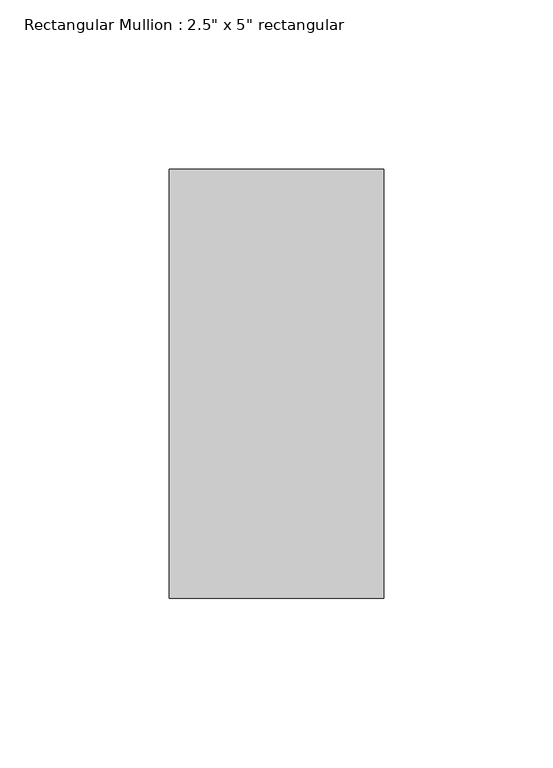
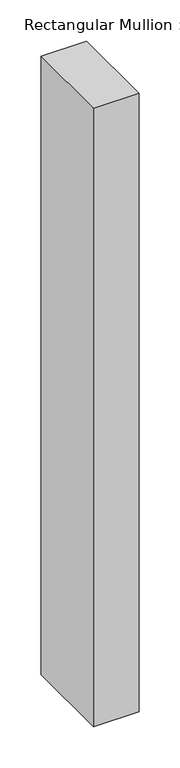
"""IFC4 building model written with IfcOpenShell, lengths in millimetres: member geometry."""

from ifc_helpers import new_model, si_unit, frame, origin, place, context, project, spatial, polyline, outline, extrude, source, transform, mapped, element, save


def member_410c6227(model_context):
    return source(origin(), model_context, "Body", "SweptSolid", [
        extrude(outline(polyline([(31.75, 63.5), (31.75, -63.5), (-31.75, -63.5), (-31.75, 63.5), (31.75, 63.5)])), frame((0.0, 0.0, -914.4), z_axis=(0.0, 0.0, 1.0), x_axis=(1.0, 0.0, 0.0)), (0.0, 0.0, 1.0), 914.4),
    ])


if __name__ == "__main__":
    model = new_model("IFC4")
    model_context = context("Model", 3, world=origin())
    ifc_project = project(units=[si_unit("LENGTHUNIT", "METRE", prefix="MILLI")], contexts=[model_context])
    site = spatial("IfcSite", under=ifc_project)
    building = spatial("IfcBuilding", under=site)
    placement = place(None, origin())
    member_shape = member_410c6227(model_context)
    element("IfcMember", 1, ObjectType="Rectangular Mullion : 2.5\" x 5\" rectangular", at=placement, inside=building, context=model_context, shape_type="MappedRepresentation", body=[
        mapped(member_shape, transform((0.0, 0.0, 0.0), x_axis=(1.0, 0.0, 0.0), y_axis=(0.0, 1.0, 0.0), z_axis=(0.0, 0.0, 1.0))),
    ])
    save(model, "model.ifc")

# Revit data of these elements
# Type "Rectangular Mullion : 2.5\" x 5\" rectangular"
#   built-in parameter 1007304 = 0.416667 (stored number, unit not read)
#   built-in parameter 1007301 = 0.104167 (stored number, unit not read)
#   built-in parameter 1007300 = 0.104167 (stored number, unit not read)
# Element 1 (IfcMember, "Rectangular Mullion : 2.5\" x 5\" rectangular")
#   Materials on its faces: "metal black"
# Materials
#   "metal black": class "Generic", colour RGB 120 120 120, transparency 0, Cost = 0
